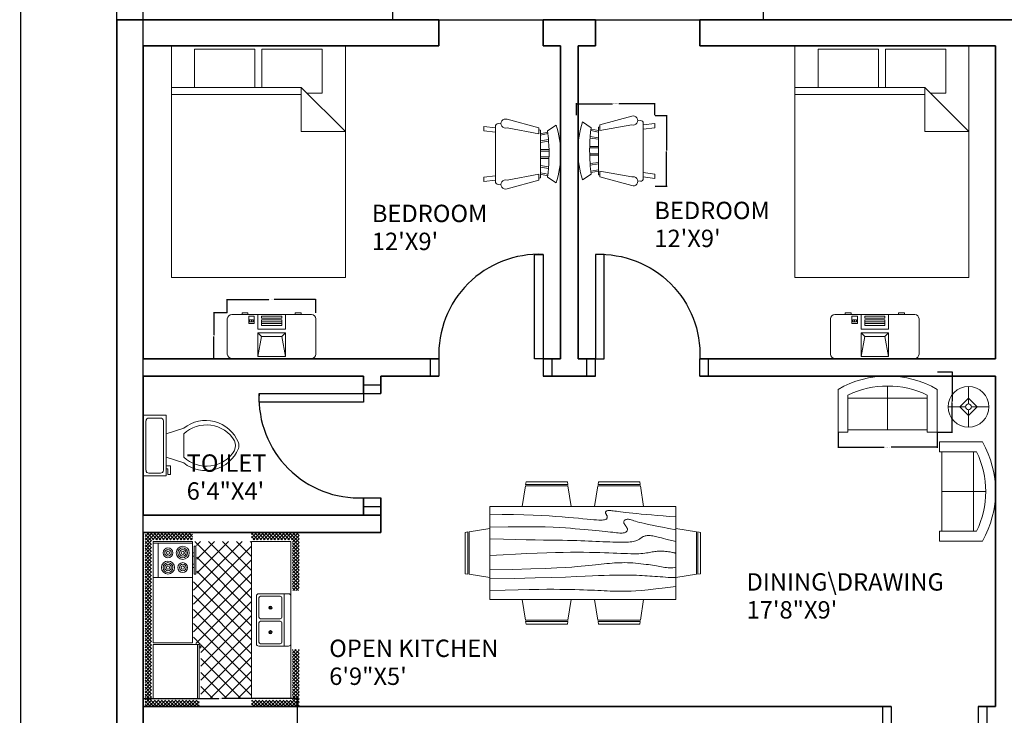
# Model space of a CAD drawing. Units: inches. Extents: x 4159 to 4826, y 299 to 1026.
# Tile 35 of 37: x 4159 to 4498, y 663 to 903. Entities that reach past the tile are written whole.
import ezdxf

# ---------------------------------------------------------------- set-up
doc = ezdxf.new("R2010")
doc.units = ezdxf.units.IN
for name, color, linetype, lineweight in [('A-ANNO-DIMS', 2, 'Continuous', 18), ('A-AREA-IDEN', 7, 'Continuous', 18), ('A-DOOR', 4, 'Continuous', 25), ('A-EQPM', 8, 'Continuous', 13), ('A-FLOR-BALC', 7, 'Continuous', 25), ('A-FLOR-FIXT', 9, 'Continuous', 18), ('A-FURN', 8, 'Continuous', 18), ('A-WALL', 7, 'Continuous', 35)]:
    doc.layers.add(name, color=color, linetype=linetype, lineweight=lineweight)
doc.styles.get("Standard").update_dxf_attribs({"font": 'arial.ttf'})
doc.dimstyles.get("Standard").update_dxf_attribs({"dimtxt": 0.18, "dimasz": 0.18, "dimexe": 0.18, "dimexo": 0.0625, "dimgap": 0.09, "dimtad": 0, "dimtih": 1, "dimtoh": 1, "dimdec": 4, "dimzin": 0, "dimdsep": 46, "dimtxsty": 'Standard', "dimcen": 0.09, "dimadec": 0, "dimazin": 0, "dimtfac": 1, "dimtdec": 4, "dimtofl": 0, "dimtmove": 0, "dimatfit": 3, "dimfxl": 1, "dimtolj": 1, "dimtzin": 0, "dimarcsym": 0})

# ---------------------------------------------------------------- blocks, each defined once
blk = doc.blocks.new('Chair - Rocking')
for p, q in [((-8, -4.5), (-10, -1.5)), ((8, -4.5), (10, -1.5)), ((-7.5, -4.5), (-7, -7)), ((-6.5, -7), (-7.02225, -4.43)), ((-4.5, -7), (-4.96674, -4.19951)), ((-4, -7), (-4.40532, -4.16272)), ((-1.5, -4.05012), (-1.5, -7)), ((-1, -7), (-1, -4.05012)), ((1, -7), (1, -4.04655)), ((1.5, -4.05012), (1.5, -7)), ((4, -7), (4.40187, -4.18694)), ((4.5, -7), (4.96761, -4.19437)), ((6.5, -7), (7, -4.4057)), ((7.5, -4.5), (7, -7)), ((-9, -7.5), (-12, -18.49999)), ((-7, -7.5), (-9, -7.5)), ((-9, -18.49999), (-7, -7.5)), ((-8.23428, -6.99939), (-8.3093, -7.47958)), ((-8.23041, -7), (8.23915, -7)), ((7, -7.5), (9, -7.5)), ((9, -18.49999), (7, -7.5)), ((8.31071, -7.48854), (8.23449, -7.00073)), ((9, -7.5), (12, -18.49999)), ((-10.36644, -20.64523), (-10.5, -21.49999)), ((-9, -22.49999), (-9.5, -26.49999)), ((0, -22.49999), (-9.5, -22.49999)), ((-8, -26.49999), (-7.5, -22.49999)), ((0, -22.49999), (9.5, -22.49999)), ((8, -26.49999), (7.5, -22.49999)), ((9, -22.49999), (9.5, -26.49999)), ((10.5, -21.49999), (10.3575, -20.58798)), ((-9.5, -26.49999), (-8, -26.49999)), ((9.5, -26.49999), (8, -26.49999))]:
    blk.add_line(p, q)
for centre, radius, start, end in [((0, -34.08333), 34.08333, 72.93847, 107.0615), ((0, -68.25004), 64.25, 93.92211, 97.15267), ((0, -68.25004), 64.25, 82.84733, 93.92211), ((-10.5, -18.99999), 1.58114, 161.5651, 18.43495), ((10.5, -18.99999), 1.58114, 161.5651, 18.43495), ((-9.5, -21.49999), 1, 180, 270), ((9.5, -21.49999), 1, 270, 0)]:
    blk.add_arc(centre, radius, start, end)
blk = doc.blocks.new('Bed - Queen')
for p, q in [((0, -80.00003), (0, 0)), ((0, 0), (59.99999, 0)), ((59.99999, 0), (59.99999, -80.00003)), ((7.99999, -1.2), (28.79998, -1.2)), ((7.99999, -14.4), (7.99999, -1.2)), ((28.79998, -1.2), (28.79998, -14.4)), ((31.19999, -1.2), (51.99999, -1.2)), ((31.19999, -14.4), (31.19999, -1.2)), ((51.99999, -1.2), (51.99999, -16.4)), ((0, -14.4), (44.8, -14.4)), ((44.8, -16.8), (0, -16.8)), ((59.99999, -29.6), (44.8, -14.4)), ((44.8, -14.4), (44.8, -29.6)), ((51.99999, -16.4), (46.79936, -16.4)), ((44.8, -29.6), (59.99999, -29.6)), ((59.99999, -80.00003), (0, -80.00003))]:
    blk.add_line(p, q)
blk = doc.blocks.new('Dining Set - 36 x 72 in.')
for p, q in [((-22, 27.5), (-22.1562, 26.50042)), ((-22, 27.5), (-6, 27.5)), ((-5.8437, 26.49966), (-6, 27.5)), ((6, 27.5), (5.8438, 26.50042)), ((6, 27.5), (22, 27.5)), ((22.1563, 26.49966), (22, 27.5)), ((-22.2343, 26.00059), (-23.4847, 17.99762)), ((-22.2304, 26), (-5.7608, 26)), ((-5.8416, 26.5), (-22.1534, 26.5)), ((-4.5152, 17.99762), (-5.7655, 25.99926)), ((5.7657, 26.00059), (4.5153, 17.99762)), ((5.7696, 26), (22.2392, 26)), ((22.1584, 26.5), (5.8466, 26.5)), ((23.4848, 17.99762), (22.2345, 25.99926)), ((36, 18), (-36, 18)), ((-36, 18), (-36, -18)), ((36, -18), (36, 18)), ((-45.5, 8), (-44.5004, 8.15617)), ((-45.5, 8), (-45.5, -8)), ((-44.5, -8.15843), (-44.5, 8.15338)), ((-44.0006, 8.23428), (-35.9976, 9.48474)), ((-44, 8.23041), (-44, -8.23915)), ((44.0006, 8.23428), (35.9976, 9.48474)), ((44, 8.23041), (44, -8.23915)), ((44.5, -8.15843), (44.5, 8.15338)), ((45.5, 8), (44.5005, 8.15617)), ((45.5, 8), (45.5, -8)), ((-44.4997, -8.15631), (-45.5, -8)), ((-35.9976, -9.48476), (-43.9993, -8.2345)), ((35.9976, -9.48476), (43.9993, -8.2345)), ((44.4997, -8.15631), (45.5, -8)), ((-36, -18), (36, -18)), ((-22.2343, -26.0006), (-23.4847, -17.99762)), ((-4.5152, -17.99762), (-5.7655, -25.99928)), ((5.7657, -26.0006), (4.5153, -17.99762)), ((23.4848, -17.99762), (22.2345, -25.99928)), ((-22.2304, -26), (-5.7608, -26)), ((-22, -27.5), (-22.1562, -26.50044)), ((-5.8416, -26.5), (-22.1534, -26.5)), ((-5.8437, -26.49967), (-6, -27.5)), ((5.7696, -26), (22.2392, -26)), ((6, -27.5), (5.8438, -26.50044)), ((22.1584, -26.5), (5.8466, -26.5)), ((22.1563, -26.49967), (22, -27.5)), ((-22, -27.5), (-6, -27.5)), ((6, -27.5), (22, -27.5))]:
    blk.add_line(p, q)
for points in [[(-36, 15), (-31.1772, 14.97754), (-26.8079, 14.91406), (-22.8538, 14.81543), (-19.276, 14.6875), (-16.0362, 14.53613), (-13.0957, 14.36718), (-10.4159, 14.18652), (-7.9583, 14), (-5.6904, 13.81315), (-3.6035, 13.63021), (-1.6954, 13.45508), (0.0365, 13.29166), (1.5945, 13.14388), (2.9811, 13.01562), (4.1988, 12.9108), (5.25, 12.83333), (6.1393, 12.78613), (6.8802, 12.76823), (7.4883, 12.77767), (7.9792, 12.8125), (8.3685, 12.87077), (8.6719, 12.95052), (8.9049, 13.0498), (9.0833, 13.16666), (9.2205, 13.29899), (9.3216, 13.44401), (9.3895, 13.59879), (9.4271, 13.76041), (9.4373, 13.92594), (9.4232, 14.09245), (9.3875, 14.257), (9.3333, 14.41666), (9.2638, 14.56917), (9.1836, 14.71484), (9.0975, 14.85465), (9.0104, 14.98958), (8.9272, 15.1206), (8.8529, 15.2487), (8.7922, 15.37483), (8.75, 15.5), (8.7305, 15.62467), (8.7344, 15.74739), (8.7617, 15.86621), (8.8125, 15.97916), (8.8867, 16.08431), (8.9844, 16.17968), (9.1055, 16.26334), (9.25, 16.33333), (9.4189, 16.38802), (9.6172, 16.42708), (9.8506, 16.45052), (10.125, 16.45833), (10.4463, 16.45052), (10.8203, 16.42708), (11.2529, 16.38802), (11.75, 16.33333), (12.3184, 16.26318), (12.9694, 16.17838), (13.7151, 16.07991), (14.5677, 15.96875), (15.5395, 15.84586), (16.6426, 15.71224), (17.8893, 15.56884), (19.2917, 15.41666), (20.859, 15.25667), (22.5879, 15.08984), (24.4721, 14.91715), (26.5052, 14.73958), (28.6809, 14.5581), (30.9929, 14.3737), (33.4347, 14.18733), (36, 14)], [(-36, 10), (-28.9766, 10.14274), (-23.1725, 10.20442), (-18.4241, 10.19775), (-14.5677, 10.13541), (-11.4399, 10.03011), (-8.877, 9.89453), (-6.7154, 9.74137), (-4.7917, 9.58333), (-2.9698, 9.43082), (-1.2246, 9.28515), (0.4415, 9.14534), (2.026, 9.01041), (3.5266, 8.87939), (4.9408, 8.7513), (6.266, 8.62516), (7.5, 8.5), (8.6411, 8.37549), (9.6914, 8.2539), (10.6538, 8.13818), (11.5312, 8.03125), (12.3267, 7.93603), (13.043, 7.85547), (13.6831, 7.79248), (14.25, 7.75), (14.7471, 7.7303), (15.1797, 7.73307), (15.5537, 7.75732), (15.875, 7.80208), (16.1494, 7.86637), (16.3828, 7.94922), (16.5811, 8.04964), (16.75, 8.16666), (16.8944, 8.29915), (17.0143, 8.44531), (17.1089, 8.60319), (17.1771, 8.77083), (17.218, 8.94629), (17.2305, 9.1276), (17.2137, 9.31282), (17.1667, 9.5), (17.0895, 9.6875), (16.987, 9.875), (16.8649, 10.0625), (16.7292, 10.25), (16.5856, 10.4375), (16.4401, 10.625), (16.2985, 10.8125), (16.1667, 11), (16.05, 11.18733), (15.9518, 11.3737), (15.8752, 11.5581), (15.8229, 11.73958), (15.798, 11.91715), (15.8034, 12.08984), (15.842, 12.25667), (15.9167, 12.41666), (16.0295, 12.56836), (16.1784, 12.70833), (16.3605, 12.83268), (16.5729, 12.9375), (16.8127, 13.01888), (17.0768, 13.07291), (17.3625, 13.0957), (17.6667, 13.08333), (17.9894, 13.03312), (18.3418, 12.94726), (18.7382, 12.82918), (19.1927, 12.68229), (19.7195, 12.51001), (20.3327, 12.31575), (21.0465, 12.10294), (21.875, 11.875), (22.8357, 11.63354), (23.959, 11.37304), (25.2786, 11.08618), (26.8282, 10.76562), (28.6414, 10.40405), (30.752, 9.99414), (33.1936, 9.52856), (36, 9)], [(-36, 5.5), (-30.7157, 5.3348), (-26.069, 5.20963), (-21.9946, 5.11767), (-18.4271, 5.05208), (-15.3009, 5.00602), (-12.5508, 4.97265), (-10.1112, 4.94515), (-7.9167, 4.91666), (-5.909, 4.88167), (-4.0586, 4.83984), (-2.3429, 4.79215), (-0.7396, 4.73958), (0.7739, 4.6831), (2.22, 4.6237), (3.6213, 4.56233), (5, 4.5), (6.373, 4.43782), (7.7344, 4.3776), (9.0723, 4.32129), (10.375, 4.27083), (11.6309, 4.22819), (12.8281, 4.19531), (13.9551, 4.17415), (15, 4.16666), (15.954, 4.17448), (16.819, 4.19791), (17.6001, 4.23698), (18.3021, 4.29166), (18.9299, 4.36198), (19.4883, 4.44791), (19.9823, 4.54948), (20.4167, 4.66666), (20.7969, 4.79899), (21.1302, 4.94401), (21.4245, 5.09879), (21.6875, 5.26041), (21.9271, 5.42594), (22.1511, 5.59245), (22.3672, 5.757), (22.5834, 5.91666), (22.8065, 6.06868), (23.0404, 6.21093), (23.2879, 6.34147), (23.5521, 6.45833), (23.8358, 6.55957), (24.142, 6.64323), (24.4735, 6.70735), (24.8334, 6.75), (25.2235, 6.76969), (25.642, 6.76692), (26.0858, 6.74267), (26.5521, 6.69791), (27.0379, 6.63362), (27.5404, 6.55078), (28.0565, 6.45036), (28.5834, 6.33333), (29.1242, 6.19987), (29.7071, 6.04687), (30.3661, 5.87044), (31.1354, 5.66666), (32.0493, 5.43164), (33.142, 5.16146), (34.4475, 4.85221), (36, 4.5)], [(-36, -1), (-30.7915, -0.6591), (-26.0195, -0.38216), (-21.6519, -0.16284), (-17.6563, 0.00521), (-14.0005, 0.12833), (-10.6523, 0.21289), (-7.5796, 0.26522), (-4.75, 0.29166), (-2.134, 0.29793), (0.2878, 0.28711), (2.5317, 0.26163), (4.6146, 0.22396), (6.5529, 0.17651), (8.3633, 0.12174), (10.0623, 0.06209), (11.6667, 0), (13.1899, -0.06201), (14.6341, -0.1211), (15.9982, -0.17432), (17.2813, -0.21875), (18.4823, -0.25147), (19.6003, -0.26953), (20.6343, -0.27002), (21.5834, -0.25), (22.4481, -0.20768), (23.2357, -0.14584), (23.9549, -0.06836), (24.6146, 0.02083), (25.2235, 0.11784), (25.7904, 0.21875), (26.3241, 0.31966), (26.8334, 0.41666), (27.3265, 0.50618), (27.8099, 0.58593), (28.2894, 0.65397), (28.7709, 0.70833), (29.2601, 0.74707), (29.763, 0.76823), (30.2855, 0.76985), (30.8334, 0.75), (31.4088, 0.70784), (31.9994, 0.64713), (32.589, 0.57275), (33.1615, 0.48958), (33.7008, 0.4025), (34.1908, 0.3164), (34.6153, 0.23616), (34.9584, 0.16666), (35.2099, 0.11165), (35.3848, 0.07031), (35.504, 0.04069), (35.5886, 0.02083), (35.6594, 0.00879), (35.7377, 0.0026), (35.8442, 0.00032), (36, 0)], [(-36, -6.5), (-27.1843, -6.31267), (-20.084, -6.1263), (-14.469, -5.9419), (-10.1094, -5.76042), (-6.7752, -5.58285), (-4.2363, -5.41016), (-2.2629, -5.24333), (-0.625, -5.08334), (0.8708, -4.93099), (2.2715, -4.78646), (3.5872, -4.64974), (4.8281, -4.52084), (6.0046, -4.39974), (7.127, -4.28646), (8.2053, -4.18099), (9.25, -4.08334), (10.2705, -3.99382), (11.2734, -3.91407), (12.2647, -3.84603), (13.25, -3.79167), (14.2354, -3.75293), (15.2266, -3.73177), (16.2295, -3.73015), (17.25, -3.75), (18.2912, -3.79248), (19.3451, -3.85547), (20.4009, -3.93604), (21.4479, -4.03125), (22.4754, -4.13819), (23.4727, -4.25391), (24.4289, -4.37549), (25.3334, -4.5), (26.1785, -4.62492), (26.9694, -4.74935), (27.7145, -4.87281), (28.4219, -4.99479), (29.1, -5.11483), (29.7572, -5.23242), (30.4016, -5.34709), (31.0417, -5.45834), (31.6837, -5.56437), (32.3262, -5.65821), (32.9658, -5.73153), (33.599, -5.77604), (34.2224, -5.78345), (34.8327, -5.74545), (35.4264, -5.65373), (36, -5.5)], [(-36, -10), (-26.4022, -9.81299), (-18.4675, -9.62891), (-11.9839, -9.45069), (-6.7396, -9.28125), (-2.5226, -9.12354), (0.8789, -8.98047), (3.6769, -8.85498), (6.0833, -8.75), (8.2767, -8.66765), (10.3021, -8.60677), (12.1712, -8.56543), (13.8958, -8.54167), (15.4876, -8.53353), (16.9583, -8.53907), (18.3197, -8.55632), (19.5834, -8.58334), (20.7616, -8.61841), (21.8685, -8.66081), (22.9188, -8.71004), (23.9271, -8.76563), (24.9081, -8.82707), (25.8763, -8.89388), (26.8465, -8.96558), (27.8334, -9.04167), (28.8474, -9.12118), (29.8828, -9.20117), (30.93, -9.27824), (31.9792, -9.34896), (33.0205, -9.40991), (34.0443, -9.45768), (35.0407, -9.48885), (36, -9.5)], [(-36, -14.5), (-30.0881, -14.33513), (-25.0332, -14.21224), (-20.7312, -14.12647), (-17.0781, -14.07292), (-13.97, -14.04671), (-11.3027, -14.04297), (-8.9724, -14.05681), (-6.875, -14.08334), (-4.9224, -14.11833), (-3.0905, -14.16016), (-1.3709, -14.20785), (0.2448, -14.26042), (1.7647, -14.3169), (3.1973, -14.3763), (4.5507, -14.43767), (5.8333, -14.5), (7.0554, -14.5621), (8.235, -14.62175), (9.3922, -14.67652), (10.5469, -14.72396), (11.7192, -14.76164), (12.929, -14.78711), (14.1965, -14.79794), (15.5417, -14.79167), (16.9933, -14.76424), (18.6152, -14.70508), (20.4804, -14.60197), (22.6615, -14.44271), (25.2312, -14.21509), (28.2624, -13.9069), (31.8277, -13.50594), (36, -13)]]:
    blk.add_lwpolyline(points)
blk = doc.blocks.new('Sofa - Roundback Loveseat 5 ft.')
for p, q in [((-24, -33.99998), (-24, -11.46958)), ((0, -32.44198), (0, -5.99998)), ((24.00004, -33.99998), (24.00004, -11.46958)), ((-23.9998, -13.38178), (23.99986, -13.38178)), ((-24, -32.44198), (24.00004, -32.44198))]:
    blk.add_line(p, q)
for points in [[(-24, -33.99998), (-30, -33.99998), (-30, -7.99998)], [(30.00004, -7.99998), (30.00004, -33.99998), (24.00004, -33.99998)]]:
    blk.add_lwpolyline(points)
for centre, radius, start, end in [((0, -60.24998), 60.24998, 60.13715, 119.8628), ((0, -61.38438), 55.38444, 64.32083, 115.6792)]:
    blk.add_arc(centre, radius, start, end)
blk = doc.blocks.new('Toilet - top')
for p, q in [((9.5, -6), (9.5, -2)), ((-10, -8.5), (-8, -8.5)), ((-10, -9.5), (-10, -8.5)), ((-7, -9.5), (-10, -9.5)), ((-8, -8.5), (-8, -8)), ((-7, -8), (-7, -9.5)), ((-4, -8), (-6, -14)), ((4, -8), (6, -14)), ((4, -14), (-4, -14))]:
    blk.add_line(p, q)
blk.add_lwpolyline([(10.5, -8), (10.5, 0), (-10.5, 0), (-10.5, -8)], close=True)
for points in [[(-9.5, -2), (-9.5, -6)], [(8.5, -1), (-8.5, -1)], [(-8.5, -7), (8.5, -7)]]:
    blk.add_lwpolyline(points)
for centre, radius, start, end in [((-8.62, -1.88), 0.884, 81.8699, 188.1301), ((8.62, -1.88), 0.884, 351.8699, 98.1301), ((-8.62, -6.12), 0.884, 171.8699, 278.1301), ((8.62, -6.12), 0.884, 261.8699, 8.1301), ((3.52, -21.58), 12.17, 141.4691, 247.9714), ((4.2, -21.82), 11.33, 136.3677, 238.9468), ((-3.52, -21.58), 12.17, 292.0284, 38.5307), ((-4.2, -21.82), 11.33, 301.053, 43.6321), ((0, -27.88), 4, 245.7318, 294.2682), ((0, -29), 4, 254.8605, 285.1395)]:
    blk.add_arc(centre, radius, start, end)
blk = doc.blocks.new('Lamp - Table')
for p, q in [((0, 7), (0, 1)), ((-1, 0), (-7, 0)), ((0, 3), (-3, 0)), ((-3, 0), (0, -3)), ((3, 0), (0, 3)), ((0, -3), (3, 0)), ((1, 0), (7, 0)), ((0, -1), (0, -7))]:
    blk.add_line(p, q)
for radius in [7, 1]:
    blk.add_circle((0, 0), radius)
blk = doc.blocks.new('Kitchen Layout - 7 x 8 ft')
for p, q in [((-5, 81.32), (2.68, 89)), ((-5, 83.44), (0.56, 89)), ((-5, 85.56), (-1.56, 89)), ((-5, 87.68), (-3.68, 89)), ((-1, 84.97), (-5, 88.97)), ((-1, 82.85), (-5, 86.85)), ((-1, 80.73), (-5, 84.73)), ((1.09, 85), (-2.91, 89)), ((3.21, 85), (-0.79, 89)), ((0.81, 85), (4.81, 89)), ((5.34, 85), (1.34, 89)), ((2.93, 85), (6.93, 89)), ((7.46, 85), (3.46, 89)), ((5.05, 85), (9.05, 89)), ((9.58, 85), (5.58, 89)), ((7.17, 85), (11.17, 89)), ((11.7, 85), (7.7, 89)), ((9.29, 85), (13.29, 89)), ((13.82, 85), (9.82, 89)), ((11.41, 85), (15.41, 89)), ((15.94, 85), (11.94, 89)), ((13.53, 85), (17.53, 89)), ((18.06, 85), (14.06, 89)), ((15.65, 85), (19.65, 89)), ((20.18, 85), (16.18, 89)), ((17.78, 85), (21.78, 89)), ((22.31, 85), (18.31, 89)), ((19.9, 85), (23.9, 89)), ((24.43, 85), (20.43, 89)), ((22.02, 85), (26.02, 89)), ((26.55, 85), (22.55, 89)), ((24.14, 85), (28.14, 89)), ((28.67, 85), (24.67, 89)), ((26.26, 85), (30.26, 89)), ((30.79, 85), (26.79, 89)), ((28.38, 85), (32.38, 89)), ((32.91, 85), (28.91, 89)), ((30.5, 85), (34.5, 89)), ((35.03, 85), (31.03, 89)), ((32.63, 85), (36.63, 89)), ((37.16, 85), (33.16, 89)), ((34.75, 85), (38.75, 89)), ((39.28, 85), (35.28, 89)), ((36.87, 85), (40.87, 89)), ((41.4, 85), (37.4, 89)), ((38.99, 85), (42.99, 89)), ((43.52, 85), (39.52, 89)), ((41.11, 85), (45.11, 89)), ((45.64, 85), (41.64, 89)), ((43.23, 85), (47.23, 89)), ((47.76, 85), (43.76, 89)), ((45.35, 85), (49.35, 89)), ((49.88, 85), (45.88, 89)), ((47.47, 85), (51.47, 89)), ((52, 85), (48, 89)), ((49.6, 85), (53.6, 89)), ((54.13, 85), (50.13, 89)), ((51.72, 85), (55.72, 89)), ((56.25, 85), (52.25, 89)), ((53.84, 85), (57.84, 89)), ((58.37, 85), (54.37, 89)), ((55.96, 85), (59.96, 89)), ((60.49, 85), (56.49, 89)), ((58.08, 85), (62.08, 89)), ((62.61, 85), (58.61, 89)), ((60.2, 85), (64.2, 89)), ((64.73, 85), (60.73, 89)), ((62.32, 85), (66.32, 89)), ((66.85, 85), (62.85, 89)), ((64.45, 85), (68.45, 89)), ((68.97, 85), (64.97, 89)), ((66.57, 85), (70.57, 89)), ((71.1, 85), (67.1, 89)), ((68.69, 85), (72.69, 89)), ((73.22, 85), (69.22, 89)), ((70.81, 85), (74.81, 89)), ((75.34, 85), (71.34, 89)), ((72.93, 85), (76.93, 89)), ((77.46, 85), (73.46, 89)), ((75.05, 85), (79.05, 89)), ((79.58, 85), (75.58, 89)), ((77.17, 85), (81.17, 89)), ((81.7, 85), (77.7, 89)), ((79.29, 85), (83.29, 89)), ((83.82, 85), (79.82, 89)), ((81.42, 85), (85.42, 89)), ((85.95, 85), (81.95, 89)), ((83.54, 85), (87.54, 89)), ((88.07, 85), (84.07, 89)), ((85.66, 85), (89.66, 89)), ((90.19, 85), (86.19, 89)), ((87.78, 85), (91.78, 89)), ((92.31, 85), (88.31, 89)), ((89.9, 85), (93.9, 89)), ((94.43, 85), (90.43, 89)), ((92.02, 85), (96.02, 89)), ((96.55, 85), (92.55, 89)), ((94.14, 85), (98.14, 89)), ((101, 82.67), (94.67, 89)), ((96.27, 85), (100.27, 89)), ((101, 84.79), (96.79, 89)), ((97, 83.61), (101, 87.61)), ((97, 81.49), (101, 85.49)), ((101, 80.55), (97, 84.55)), ((101, 86.92), (98.92, 89)), ((-5, 79.19), (-1, 83.19)), ((-1, 78.61), (-5, 82.61)), ((-5, 77.07), (-1, 81.07)), ((-1, 76.49), (-5, 80.49)), ((-5, 74.95), (-1, 78.95)), ((-1, 74.36), (-5, 78.36)), ((34, 84), (96, 84)), ((34, 60), (34, 84)), ((74, 81), (95, 81)), ((96, 84), (96, 60)), ((97, 79.37), (101, 83.37)), ((101, 78.43), (97, 82.43)), ((97, 77.25), (101, 81.25)), ((101, 76.31), (97, 80.31)), ((97, 75.13), (101, 79.13)), ((101, 74.19), (97, 78.19)), ((-5, 72.83), (-1, 76.83)), ((-1, 72.24), (-5, 76.24)), ((-5, 70.71), (-1, 74.71)), ((-1, 70.12), (-5, 74.12)), ((-5, 68.59), (-1, 72.59)), ((97, 73.01), (101, 77.01)), ((101, 72.07), (97, 76.07)), ((97, 70.89), (101, 74.89)), ((101, 69.95), (97, 73.95)), ((97, 68.76), (101, 72.76)), ((-1, 68), (-5, 72)), ((-5, 66.47), (-1, 70.47)), ((-1, 65.88), (-5, 69.88)), ((-5, 64.35), (-1, 68.35)), ((-1, 63.76), (-5, 67.76)), ((-5, 62.22), (-1, 66.22)), ((101, 67.82), (97, 71.82)), ((97, 66.64), (101, 70.64)), ((101, 65.7), (97, 69.7)), ((97, 64.52), (101, 68.52)), ((101, 63.58), (97, 67.58)), ((97, 62.4), (101, 66.4)), ((-1, 61.64), (-5, 65.64)), ((-5, 60.1), (-1, 64.1)), ((-1, 59.52), (-5, 63.52)), ((-5, 57.98), (-1, 61.98)), ((-1, 57.39), (-5, 61.39)), ((101, 61.46), (97, 65.46)), ((97, 60.28), (101, 64.28)), ((100.34, 60), (97, 63.34)), ((98.22, 60), (97, 61.22)), ((98.84, 60), (101, 62.16)), ((-1.73, 56), (-5, 59.27)), ((-3.85, 56), (-5, 57.15)), ((-4.86, 56), (-1, 59.86)), ((-2.74, 56), (-1, 57.74)), ((0, 57), (33, 57)), ((0, 30.57), (24.43, 55)), ((0, 39.06), (15.94, 55)), ((0, 47.54), (7.46, 55)), ((1.91, 24), (32.91, 55)), ((33.77, 24), (2.77, 55)), ((10.4, 24), (45.9, 59.5)), ((42.26, 24), (11.26, 55)), ((18.88, 24), (54.38, 59.5)), ((50.74, 24), (19.74, 55)), ((27.37, 24), (62.87, 59.5)), ((59.23, 24), (28.23, 55)), ((31, 55), (31, 56)), ((32, 55), (31, 55)), ((32, 56), (32, 55)), ((33.03, 55.11), (37.41, 59.5)), ((67.71, 24), (33.68, 58.04)), ((96, 60), (34, 60)), ((35.85, 24), (71.35, 59.5)), ((76.2, 24), (40.7, 59.5)), ((44.34, 24), (77.84, 57.5)), ((84.68, 24), (49.18, 59.5)), ((52.82, 24), (86.32, 57.5)), ((93.17, 24), (57.67, 59.5)), ((61.31, 24), (96, 58.69)), ((96, 29.65), (66.15, 59.5)), ((96, 38.14), (76.64, 57.5)), ((80, 60), (80, 59)), ((82, 59), (82, 60)), ((96, 46.63), (85.13, 57.5)), ((87, 59), (87, 60)), ((89, 60), (89, 59)), ((96, 55.11), (93.57, 57.54)), ((100.96, 60), (101, 60.04)), ((25.29, 24), (0, 49.29)), ((69.79, 24), (96, 50.21)), ((16.8, 24), (0, 40.8)), ((78.28, 24), (96, 41.72)), ((8.32, 24), (0, 32.32)), ((86.76, 24), (96, 33.24)), ((95.25, 24), (96, 24.75)), ((-5, 21.92), (-2.92, 24)), ((-5, 19.8), (-1, 23.8)), ((-1, 19.21), (-5, 23.21)), ((-5, 17.68), (-1, 21.68)), ((-1, 17.09), (-5, 21.09)), ((-5, 15.55), (-1, 19.55)), ((-1, 14.97), (-5, 18.97)), ((-1, 21.33), (-3.67, 24)), ((-1, 23.45), (-1.55, 24)), ((0, 24), (96, 24)), ((0, 0), (0, 24)), ((47.25, 6.5), (47.25, 18.5)), ((48.75, 18.5), (48.75, 6.5)), ((96, 24), (96, 0)), ((97, 22.1), (98.9, 24)), ((97, 19.97), (101, 23.97)), ((101, 19.03), (97, 23.03)), ((97, 17.85), (101, 21.85)), ((101, 16.91), (97, 20.91)), ((97, 15.73), (101, 19.73)), ((101, 14.79), (97, 18.79)), ((101, 21.16), (98.16, 24)), ((101, 23.28), (100.28, 24)), ((-5, 13.43), (-1, 17.43)), ((-1, 12.85), (-5, 16.85)), ((-5, 11.31), (-1, 15.31)), ((-1, 10.73), (-5, 14.73)), ((-5, 9.19), (-1, 13.19)), ((-1, 8.6), (-5, 12.6)), ((97, 13.61), (101, 17.61)), ((101, 12.67), (97, 16.67)), ((97, 11.49), (101, 15.49)), ((101, 10.55), (97, 14.55)), ((97, 9.37), (101, 13.37)), ((101, 8.43), (97, 12.43)), ((-5, 7.07), (-1, 11.07)), ((-1, 6.48), (-5, 10.48)), ((-5, 4.95), (-1, 8.95)), ((-1, 4.36), (-5, 8.36)), ((-5, 2.83), (-1, 6.83)), ((-1, 2.24), (-5, 6.24)), ((97, 7.25), (101, 11.25)), ((101, 6.31), (97, 10.31)), ((97, 5.12), (101, 9.12)), ((101, 4.18), (97, 8.18)), ((97, 3), (101, 7)), ((101, 2.06), (97, 6.06)), ((-5, 0.71), (-1, 4.71)), ((-1, 0.12), (-5, 4.12)), ((-5, -1.42), (-1, 2.58)), ((2, -5), (-5, 2)), ((-5, -3.54), (-1, 0.46)), ((96, 0), (0, 0)), ((64, 4), (32, 4)), ((93.24, -5), (101, 2.76)), ((95.36, -5), (101, 0.64)), ((97, 0.88), (101, 4.88)), ((101, -0.06), (97, 3.94)), ((101, -2.18), (97, 1.82)), ((-0.12, -5), (-5, -0.12)), ((-2.25, -5), (-5, -2.25)), ((-4.37, -5), (-5, -4.37)), ((-4.34, -5), (-0.34, -1)), ((-2.22, -5), (1.78, -1)), ((-0.1, -5), (3.9, -1)), ((4.12, -5), (0.12, -1)), ((2.02, -5), (6.02, -1)), ((6.24, -5), (2.24, -1)), ((4.14, -5), (8.14, -1)), ((8.36, -5), (4.36, -1)), ((6.27, -5), (10.27, -1)), ((10.48, -5), (6.48, -1)), ((8.39, -5), (12.39, -1)), ((12.6, -5), (8.6, -1)), ((10.51, -5), (14.51, -1)), ((14.73, -5), (10.73, -1)), ((12.63, -5), (16.63, -1)), ((16.85, -5), (12.85, -1)), ((14.75, -5), (18.75, -1)), ((18.97, -5), (14.97, -1)), ((16.87, -5), (20.87, -1)), ((21.09, -5), (17.09, -1)), ((18.99, -5), (22.99, -1)), ((23.21, -5), (19.21, -1)), ((21.11, -5), (25.11, -1)), ((25.33, -5), (21.33, -1)), ((23.24, -5), (27.24, -1)), ((27.45, -5), (23.45, -1)), ((25.36, -5), (29.36, -1)), ((29.57, -5), (25.57, -1)), ((27.48, -5), (30, -2.48)), ((30, -3.3), (27.7, -1)), ((29.6, -5), (30, -4.6)), ((30, -1.18), (29.82, -1)), ((66, -2.54), (67.54, -1)), ((66, -4.66), (69.66, -1)), ((69.88, -5), (66, -1.12)), ((67.76, -5), (66, -3.24)), ((67.78, -5), (71.78, -1)), ((72, -5), (68, -1)), ((69.9, -5), (73.9, -1)), ((74.12, -5), (70.12, -1)), ((72.03, -5), (76.03, -1)), ((76.24, -5), (72.24, -1)), ((74.15, -5), (78.15, -1)), ((78.36, -5), (74.36, -1)), ((76.27, -5), (80.27, -1)), ((80.49, -5), (76.49, -1)), ((78.39, -5), (82.39, -1)), ((82.61, -5), (78.61, -1)), ((80.51, -5), (84.51, -1)), ((84.73, -5), (80.73, -1)), ((82.63, -5), (86.63, -1)), ((86.85, -5), (82.85, -1)), ((84.75, -5), (88.75, -1)), ((88.97, -5), (84.97, -1)), ((86.88, -5), (90.88, -1)), ((91.09, -5), (87.09, -1)), ((89, -5), (93, -1)), ((93.21, -5), (89.21, -1)), ((91.12, -5), (95.12, -1)), ((95.34, -5), (91.34, -1)), ((97.46, -5), (93.46, -1)), ((99.58, -5), (95.58, -1)), ((101, -4.3), (97, -0.3)), ((97.48, -5), (101, -1.48)), ((99.6, -5), (101, -3.6))]:
    blk.add_line(p, q)
for points in [[(0, 56), (0, 84), (33, 84), (33, 56)], [(74, 60), (74, 84), (95, 84), (95, 60)], [(76, 58), (76, 59), (93, 59), (93, 58)]]:
    blk.add_lwpolyline(points, close=True)
for points in [[(32, 1.5), (32, 19.5)], [(33.5, 21), (62.5, 21)], [(33.5, 6.5), (33.5, 18.5)], [(34.5, 19.5), (46.25, 19.5)], [(49.75, 19.5), (61.5, 19.5)], [(62.5, 18.5), (62.5, 6.5)], [(64, 19.5), (64, 1.5)], [(62.5, 0), (33.5, 0)], [(46.25, 5.5), (34.5, 5.5)], [(61.5, 5.5), (49.75, 5.5)]]:
    blk.add_lwpolyline(points)
for centre, radius in [((80, 75), 4), ((80, 75), 3), ((80, 75), 2), ((80, 75), 1), ((89, 75), 3), ((89, 75), 2), ((89, 75), 1), ((80, 66), 3), ((80, 66), 2), ((80, 66), 1), ((89, 66), 4), ((89, 66), 3), ((89, 66), 2), ((89, 66), 1), ((40.5, 12.5), 1), ((40.5, 12.5), 0.5), ((55.5, 12.5), 1), ((55.5, 12.5), 0.5)]:
    blk.add_circle(centre, radius)
for centre, radius, start, end in [((33.5, 19.5), 1.5, 90, 180), ((34.5, 18.5), 1, 90, 180), ((46.25, 18.5), 1, 0, 90), ((49.75, 18.5), 1, 90, 180), ((61.5, 18.5), 1, 0, 90), ((62.5, 19.5), 1.5, 0, 90), ((34.5, 6.5), 1, 180, 270), ((46.25, 6.5), 1, 270, 0), ((49.75, 6.5), 1, 180, 270), ((61.5, 6.5), 1, 270, 0), ((33.5, 1.5), 1.5, 180, 270), ((62.5, 1.5), 1.5, 270, 0)]:
    blk.add_arc(centre, radius, start, end)
blk = doc.blocks.new('Desk - 30 x 60 in.')
for p, q in [((-26.999995, 0), (26.999995, 0)), ((-29.999995, -27), (-29.999995, -3)), ((29.999995, -3), (29.999995, -27)), ((26.999995, -30), (-26.999995, -30)), ((-20.000005, -30), (-20.000005, -31)), ((-20.000005, -31), (-16.000005, -31)), ((-16.000005, -31), (-16.000005, -30)), ((15.999995, -31), (15.999995, -30)), ((19.999995, -31), (15.999995, -31)), ((19.999995, -30), (19.999995, -31))]:
    blk.add_line(p, q)
for centre, start, end in [((-26.499995, -3.5), 98.1301, 171.8699), ((26.499995, -3.5), 8.130102, 81.8699), ((-26.499995, -26.5), 188.1301, 261.8699), ((26.499995, -26.5), 278.1301, 351.8699)]:
    blk.add_arc(centre, 3.535534, start, end)
blk = doc.blocks.new('Computer Terminal')
for p, q in [((-10, 11.5), (5, 11.5)), ((-8, 0.5), (-10, 11.5)), ((-10, -1.5), (-10, 11.5)), ((5, 11.5), (3, 0.5)), ((5, 11.5), (5, -1.5)), ((-10, -1.5), (-8, 0.5)), ((3, 0.5), (-8, 0.5)), ((3, 0.5), (5, -1.5)), ((5, -1.5), (-10, -1.5)), ((-10, -11.5), (-10, -3.5)), ((-10, -3.5), (5, -3.5)), ((5, -3.5), (5, -11.5)), ((-8, -5.5), (-8, -8.5)), ((3, -5.5), (-8, -5.5)), ((3, -6.5), (-8, -6.5)), ((-8, -7.5), (3, -7.5)), ((-8, -8.5), (3, -8.5)), ((-8, -9.5), (-8, -10.5)), ((3, -9.5), (-8, -9.5)), ((-8, -10.5), (3, -10.5)), ((3, -8.5), (3, -5.5)), ((3, -10.5), (3, -9.5)), ((10, -6.5), (7, -6.5)), ((7, -6.5), (7, -10.5)), ((7, -10.5), (10, -10.5)), ((9.5, -7.5), (7.5, -7.5)), ((7.5, -7.5), (7.5, -8.5)), ((7.5, -8.5), (9.5, -8.5)), ((8.5, -7.5), (8.5, -8.5)), ((9.5, -8.5), (9.5, -7.5)), ((10, -10.5), (10, -6.5)), ((5, -11.5), (-10, -11.5))]:
    blk.add_line(p, q)
blk = doc.blocks.new('DOOR-SWING-36IN')
blk.add_lwpolyline([(0, 0), (-3, 0), (-3, 36), (0, 36)], close=True)
blk.add_arc((-1.5, 1.5), 34.53, 87.5104, 182.4896)
blk = doc.blocks.new('DOOR-FRAME-36IN')
for p, q in [((0, 6), (0, 0)), ((3, 6), (3, 0)), ((39, 6), (39, 0)), ((42, 6), (42, 0))]:
    blk.add_line(p, q)
blk = doc.blocks.new('DOOR-FRAME-30IN')
for p, q in [((0, 6), (0, 0)), ((3, 6), (3, 0)), ((33, 6), (33, 0)), ((36, 6), (36, 0))]:
    blk.add_line(p, q)
blk = doc.blocks.new('*D25')
at = {"layer": 'A-ANNO-DIMS', "color": 0, "lineweight": -2, "transparency": 16777216}
for p, q in [((4440.97, 760.81), (4440.97, 755.56)), ((4475.17, 760.81), (4475.17, 755.56)), ((4441.15, 755.74), (4456.85, 755.74)), ((4474.99, 755.74), (4459.29, 755.74))]:
    blk.add_line(p, q, dxfattribs=at)
at = {"layer": 'A-ANNO-DIMS', "color": 0, "transparency": 16777216}
for points in [[(4441.15, 755.77), (4441.15, 755.71), (4440.97, 755.74)], [(4474.99, 755.77), (4474.99, 755.71), (4475.17, 755.74)]]:
    blk.add_solid(points, dxfattribs=at)
at = {"layer": 'Defpoints', "color": 0, "transparency": 16777216}
for p in [(4440.97, 760.87), (4475.17, 760.87), (4475.17, 755.74)]:
    blk.add_point(p, dxfattribs=at)
at = {"layer": 'A-ANNO-DIMS', "color": 0, "transparency": 16777216, "insert": (4458.07, 755.74), "char_height": 0.18, "attachment_point": 5}
blk.add_mtext('\\A1;LOVESEAT 34 TYP.', dxfattribs=at)
blk = doc.blocks.new('*D26')
at = {"layer": 'A-ANNO-DIMS', "color": 0, "lineweight": -2, "transparency": 16777216}
for p, q in [((4475.23, 781.77), (4480.48, 781.77)), ((4480.3, 781.59), (4480.3, 771.5)), ((4480.3, 761.05), (4480.3, 771.14)), ((4475.23, 760.87), (4480.48, 760.87))]:
    blk.add_line(p, q, dxfattribs=at)
at = {"layer": 'A-ANNO-DIMS', "color": 0, "transparency": 16777216}
for points in [[(4480.27, 781.59), (4480.33, 781.59), (4480.3, 781.77)], [(4480.27, 761.05), (4480.33, 761.05), (4480.3, 760.87)]]:
    blk.add_solid(points, dxfattribs=at)
at = {"layer": 'Defpoints', "color": 0, "transparency": 16777216}
for p in [(4475.17, 781.77), (4480.3, 781.77), (4475.17, 760.87)]:
    blk.add_point(p, dxfattribs=at)
at = {"layer": 'A-ANNO-DIMS', "color": 0, "transparency": 16777216, "insert": (4480.3, 771.32), "char_height": 0.18, "attachment_point": 5}
blk.add_mtext('\\A1;21 TYP.', dxfattribs=at)
blk = doc.blocks.new('*D27')
at = {"layer": 'A-ANNO-DIMS', "color": 0, "lineweight": -2, "transparency": 16777216}
for p, q in [((4230.34, 802.12), (4230.34, 806.83)), ((4230.52, 806.65), (4244.73, 806.65)), ((4260.75, 806.65), (4246.53, 806.65)), ((4260.93, 802.12), (4260.93, 806.83))]:
    blk.add_line(p, q, dxfattribs=at)
at = {"layer": 'A-ANNO-DIMS', "color": 0, "transparency": 16777216}
for points in [[(4230.52, 806.68), (4230.52, 806.62), (4230.34, 806.65)], [(4260.75, 806.68), (4260.75, 806.62), (4260.93, 806.65)]]:
    blk.add_solid(points, dxfattribs=at)
at = {"layer": 'Defpoints', "color": 0, "transparency": 16777216}
for p in [(4230.34, 806.65), (4230.34, 802.06), (4260.93, 802.06)]:
    blk.add_point(p, dxfattribs=at)
at = {"layer": 'A-ANNO-DIMS', "color": 0, "transparency": 16777216, "insert": (4245.63, 806.65), "char_height": 0.18, "attachment_point": 5}
blk.add_mtext('\\A1;DESK 31 TYP.', dxfattribs=at)
blk = doc.blocks.new('*D28')
at = {"layer": 'A-ANNO-DIMS', "color": 0, "lineweight": -2, "transparency": 16777216}
for p, q in [((4230.27, 802.06), (4225.57, 802.06)), ((4225.75, 801.88), (4225.75, 794.34)), ((4225.75, 786.43), (4225.75, 793.98)), ((4230.27, 786.25), (4225.57, 786.25))]:
    blk.add_line(p, q, dxfattribs=at)
at = {"layer": 'A-ANNO-DIMS', "color": 0, "transparency": 16777216}
for points in [[(4225.72, 801.88), (4225.78, 801.88), (4225.75, 802.06)], [(4225.72, 786.43), (4225.78, 786.43), (4225.75, 786.25)]]:
    blk.add_solid(points, dxfattribs=at)
at = {"layer": 'Defpoints', "color": 0, "transparency": 16777216}
for p in [(4230.34, 802.06), (4225.75, 786.25), (4230.34, 786.25)]:
    blk.add_point(p, dxfattribs=at)
at = {"layer": 'A-ANNO-DIMS', "color": 0, "transparency": 16777216, "insert": (4225.75, 794.16), "char_height": 0.18, "attachment_point": 5}
blk.add_mtext('\\A1;16 TYP.', dxfattribs=at)
blk = doc.blocks.new('*D31')
at = {"layer": 'A-ANNO-DIMS', "color": 0, "lineweight": -2, "transparency": 16777216}
for p, q in [((4350.81, 870.26), (4350.81, 874.43)), ((4350.99, 874.25), (4363.21, 874.25)), ((4377.63, 874.25), (4365.41, 874.25)), ((4377.81, 870.26), (4377.81, 874.43))]:
    blk.add_line(p, q, dxfattribs=at)
at = {"layer": 'A-ANNO-DIMS', "color": 0, "transparency": 16777216}
for points in [[(4350.99, 874.28), (4350.99, 874.22), (4350.81, 874.25)], [(4377.63, 874.28), (4377.63, 874.22), (4377.81, 874.25)]]:
    blk.add_solid(points, dxfattribs=at)
at = {"layer": 'Defpoints', "color": 0, "transparency": 16777216}
for p in [(4350.81, 874.25), (4350.81, 870.2), (4377.81, 870.2)]:
    blk.add_point(p, dxfattribs=at)
at = {"layer": 'A-ANNO-DIMS', "color": 0, "transparency": 16777216, "insert": (4364.31, 874.25), "char_height": 0.18, "attachment_point": 5}
blk.add_mtext('\\A1;ROCKER 27 TYP.', dxfattribs=at)
blk = doc.blocks.new('*D32')
at = {"layer": 'A-ANNO-DIMS', "color": 0, "lineweight": -2, "transparency": 16777216}
for p, q in [((4377.87, 870.2), (4382.04, 870.2)), ((4381.86, 870.02), (4381.86, 858.16)), ((4381.86, 845.94), (4381.86, 857.8)), ((4377.87, 845.76), (4382.04, 845.76))]:
    blk.add_line(p, q, dxfattribs=at)
at = {"layer": 'A-ANNO-DIMS', "color": 0, "transparency": 16777216}
for points in [[(4381.83, 870.02), (4381.89, 870.02), (4381.86, 870.2)], [(4381.83, 845.94), (4381.89, 845.94), (4381.86, 845.76)]]:
    blk.add_solid(points, dxfattribs=at)
at = {"layer": 'Defpoints', "color": 0, "transparency": 16777216}
for p in [(4377.81, 870.2), (4381.86, 870.2), (4377.81, 845.76)]:
    blk.add_point(p, dxfattribs=at)
at = {"layer": 'A-ANNO-DIMS', "color": 0, "transparency": 16777216, "insert": (4381.86, 857.98), "char_height": 0.18, "attachment_point": 5}
blk.add_mtext('\\A1;24 TYP.', dxfattribs=at)
blk = doc.blocks.new('*D40')
at = {"layer": 'A-ANNO-DIMS', "color": 0, "lineweight": -2, "transparency": 16777216}
for p, q in [((4201.44, 660.12), (4201.44, 669.22)), ((4201.62, 669.04), (4227.47, 669.04)), ((4254.37, 669.04), (4228.52, 669.04)), ((4254.55, 660.12), (4254.55, 669.22))]:
    blk.add_line(p, q, dxfattribs=at)
at = {"layer": 'A-ANNO-DIMS', "color": 0, "transparency": 16777216}
for points in [[(4201.62, 669.07), (4201.62, 669.01), (4201.44, 669.04)], [(4254.37, 669.07), (4254.37, 669.01), (4254.55, 669.04)]]:
    blk.add_solid(points, dxfattribs=at)
at = {"layer": 'Defpoints', "color": 0, "transparency": 16777216}
for p in [(4201.44, 669.04), (4201.44, 660.06), (4254.55, 660.06)]:
    blk.add_point(p, dxfattribs=at)
at = {"layer": 'A-ANNO-DIMS', "color": 0, "transparency": 16777216, "insert": (4227.99, 669.04), "char_height": 0.18, "attachment_point": 5}
blk.add_mtext('\\A1;53 TYP.', dxfattribs=at)
blk = doc.blocks.new('*D44')
at = {"layer": 'A-ANNO-DIMS', "color": 0, "lineweight": -2, "transparency": 16777216}
for p, q in [((4287.26, 963.09), (4158.88, 963.09)), ((4159.06, 962.91), (4159.06, 647.83)), ((4159.06, 332.38), (4159.06, 647.46)), ((4447.25, 332.2), (4158.88, 332.2))]:
    blk.add_line(p, q, dxfattribs=at)
at = {"layer": 'A-ANNO-DIMS', "color": 0, "transparency": 16777216}
for points in [[(4159.03, 962.91), (4159.09, 962.91), (4159.06, 963.09)], [(4159.03, 332.38), (4159.09, 332.38), (4159.06, 332.2)]]:
    blk.add_solid(points, dxfattribs=at)
at = {"layer": 'Defpoints', "color": 0, "transparency": 16777216}
for p in [(4287.33, 963.09), (4159.06, 332.2), (4447.31, 332.2)]:
    blk.add_point(p, dxfattribs=at)
at = {"layer": 'A-ANNO-DIMS', "color": 0, "transparency": 16777216, "insert": (4159.06, 647.64), "char_height": 0.18, "attachment_point": 5}
blk.add_mtext('\\A1;630.9', dxfattribs=at)
blk = doc.blocks.new('*D50')
at = {"layer": 'A-ANNO-DIMS', "color": 0, "lineweight": -2, "transparency": 16777216}
for p, q in [((4192.31, 392.32), (4192.31, 1025.84)), ((4192.49, 1025.66), (4196.66, 1025.66)), ((4201.13, 1025.66), (4196.96, 1025.66)), ((4201.31, 401.32), (4201.31, 1025.84))]:
    blk.add_line(p, q, dxfattribs=at)
at = {"layer": 'A-ANNO-DIMS', "color": 0, "transparency": 16777216}
for points in [[(4192.49, 1025.69), (4192.49, 1025.63), (4192.31, 1025.66)], [(4201.13, 1025.69), (4201.13, 1025.63), (4201.31, 1025.66)]]:
    blk.add_solid(points, dxfattribs=at)
at = {"layer": 'Defpoints', "color": 0, "transparency": 16777216}
for p in [(4201.31, 1025.66), (4201.31, 401.25), (4192.31, 392.25)]:
    blk.add_point(p, dxfattribs=at)
at = {"layer": 'A-ANNO-DIMS', "color": 0, "transparency": 16777216, "insert": (4196.81, 1025.66), "char_height": 0.18, "attachment_point": 5}
blk.add_mtext('\\A1;9', dxfattribs=at)

msp = doc.modelspace()

# ---------------------------------------------------------------- linework, layer by layer
at = {"layer": 'A-FLOR-BALC'}
msp.add_lwpolyline([(4287.326, 903.254), (4415.251, 903.254), (4415.251, 963.093), (4287.326, 963.093)], close=True, dxfattribs=at)
at = {"layer": 'A-WALL'}
for p, q in [((4303.31, 894.254), (4303.31, 903.254)), ((4339.31, 894.254), (4339.31, 903.254)), ((4357.31, 894.254), (4357.31, 903.254)), ((4393.31, 894.254), (4393.31, 903.254)), ((4201.31, 894.254), (4201.31, 786.254)), ((4303.31, 894.254), (4201.31, 894.254)), ((4345.31, 894.254), (4339.31, 894.254)), ((4345.31, 894.254), (4345.31, 786.254)), ((4351.31, 894.254), (4351.31, 786.254)), ((4357.31, 894.254), (4351.31, 894.254)), ((4495.31, 894.254), (4393.31, 894.254)), ((4495.31, 894.254), (4495.31, 786.254)), ((4303.31, 786.254), (4201.31, 786.254)), ((4345.31, 786.254), (4339.31, 786.254)), ((4357.31, 786.254), (4351.31, 786.254)), ((4495.31, 786.254), (4393.31, 786.254)), ((4201.31, 780.254), (4201.31, 732.254)), ((4277.31, 780.254), (4201.31, 780.254)), ((4277.31, 780.254), (4277.31, 774.254)), ((4283.31, 780.254), (4283.31, 774.254)), ((4303.31, 780.254), (4283.31, 780.254)), ((4357.31, 780.254), (4339.31, 780.254)), ((4495.31, 780.254), (4393.31, 780.254)), ((4495.31, 780.254), (4495.31, 666.254)), ((4277.31, 738.254), (4277.31, 732.254)), ((4283.31, 738.254), (4283.31, 726.254)), ((4277.31, 732.254), (4201.31, 732.254)), ((4283.31, 732.254), (4201.31, 732.254)), ((4201.31, 726.254), (4201.31, 666.254)), ((4283.31, 726.254), (4201.31, 726.254)), ((4459.31, 666.254), (4201.31, 666.254)), ((4495.31, 666.254), (4489.31, 666.254))]:
    msp.add_line(p, q, dxfattribs=at)
for points in [[(4303.31, 903.254), (4192.31, 903.254), (4192.31, 392.254)], [(4357.31, 903.254), (4339.31, 903.254)], [(4603.31, 903.254), (4393.31, 903.254)]]:
    msp.add_lwpolyline(points, dxfattribs=at)

# ---------------------------------------------------------------- block references
at = {"layer": 'A-DOOR'}
for name, p in [('DOOR-SWING-36IN', (4339.31, 786.254)), ('DOOR-FRAME-36IN', (4300.31, 780.254)), ('DOOR-FRAME-30IN', (4456.31, 660.254))]:
    msp.add_blockref(name, p, dxfattribs=at)
at = {"layer": 'A-DOOR', "extrusion": (0, 0, -1), "zscale": -1}
msp.add_blockref('DOOR-SWING-36IN', (-4357.31, 786.254), dxfattribs=at)
at = {"layer": 'A-DOOR'}
for name, p, rotation in [('DOOR-FRAME-36IN', (4396.31, 786.254), 180), ('DOOR-SWING-36IN', (4277.31, 774.254), 90.00000000000104), ('DOOR-FRAME-36IN', (4283.31, 735.254), 90.00000000000026)]:
    msp.add_blockref(name, p, dxfattribs=dict(at, rotation=rotation))
at = {"layer": 'A-EQPM', "xscale": 0.6328414688201627, "yscale": 0.6328414688201627, "zscale": 0.6328414688201627, "rotation": 180}
for p in [(4244.051, 794.273), (4452.067, 794.27)]:
    msp.add_blockref('Computer Terminal', p, dxfattribs=at)
at = {"layer": 'A-FLOR-FIXT', "rotation": 90}
msp.add_blockref('Toilet - top', (4201.31, 756.293), dxfattribs=at)
at = {"layer": 'A-FLOR-FIXT', "xscale": 0.5650329326971529, "yscale": 0.5650329326971529, "zscale": 0.5650329326971529, "rotation": 90}
msp.add_blockref('Kitchen Layout - 7 x 8 ft', (4252.276, 668.991), dxfattribs=at)
at = {"layer": 'A-FURN'}
for p in [(4211.066, 894.254), (4426.112, 894.254)]:
    msp.add_blockref('Bed - Queen', p, dxfattribs=at)
for p, rotation in [((4351.31, 857.98), 90), ((4345.31, 856.9), 270)]:
    msp.add_blockref('Chair - Rocking', p, dxfattribs=dict(at, rotation=rotation))
for name, p, xscale, yscale, zscale, rotation in [('Desk - 30 x 60 in.', (4245.633, 786.254), 0.5098837128326598, 0.5098837128326598, 0.5098837128326598, 180), ('Desk - 30 x 60 in.', (4453.649, 786.251), 0.5098837128326598, 0.5098837128326598, 0.5098837128326598, 180), ('Sofa - Roundback Loveseat 5 ft.', (4495.31, 740.438), 0.5700533147329089, 0.5700533147329089, 0.5700533147329089, 269.999748957613)]:
    msp.add_blockref(name, p, dxfattribs=dict(at, xscale=xscale, yscale=yscale, zscale=zscale, rotation=rotation))
for name, p, xscale, yscale, zscale in [('Sofa - Roundback Loveseat 5 ft.', (4458.07, 780.254), 0.5700533147329089, 0.5700533147329089, 0.5700533147329089), ('Lamp - Table', (4485.972, 769.652), 1.003057144141322, 1.003057144141322, 1.003057144141322), ('Dining Set - 36 x 72 in.', (4352.983, 719.211), 0.8913588978043845, 0.8913588978043845, 0.8913588978043845)]:
    msp.add_blockref(name, p, dxfattribs=dict(at, xscale=xscale, yscale=yscale, zscale=zscale))

# ---------------------------------------------------------------- texts
at = {"layer": 'A-AREA-IDEN'}
for s, p in [('BEDROOM', (4280.196, 833.401)), ('BEDROOM', (4377.612, 834.425)), ("12'X9'", (4280.196, 823.762)), ("12'X9'", (4377.612, 824.787)), ('TOILET', (4216.335, 747.247)), ('6\'4"X4\'', (4216.335, 737.608)), ('DINING\\DRAWING', (4409.416, 706.249)), ('17\'8"X9\'', (4409.416, 696.611)), ('OPEN KITCHEN', (4265.487, 683.34)), ('6\'9"X5\'', (4265.487, 673.702))]:
    msp.add_text(s, height=6, dxfattribs=at).set_placement(p)

# ---------------------------------------------------------------- dimensions: what is measured, and where the dimension line sits
at = {"layer": 'A-ANNO-DIMS'}
dim = msp.add_linear_dim(base=(4201.31, 1025.662), p1=(4192.31, 392.254), p2=(4201.31, 401.254), dimstyle='Standard', override={"dimdec": 0, "dimlfac": 1, "dimrnd": 0, "dimzin": 0, "dimdsep": 46, "dimlunit": 2}, dxfattribs=at)
dim.commit()
dim.dimension.update_dxf_attribs({"geometry": '*D50', "text_midpoint": (4196.81, 1025.662)})
dim = msp.add_linear_dim(base=(4159.06, 332.195), p1=(4287.326, 963.093), p2=(4447.31, 332.195), angle=90, dimstyle='Standard', override={"dimdec": 1, "dimlfac": 1, "dimrnd": 0, "dimzin": 0, "dimdsep": 46, "dimlunit": 2}, dxfattribs=at)
dim.commit()
dim.dimension.update_dxf_attribs({"geometry": '*D44', "text_midpoint": (4159.06, 647.644)})
for base, p1, p2, angle, text, picture, middle in [((4350.81, 874.248), (4377.81, 870.198), (4350.81, 870.198), 180, 'ROCKER <> TYP.', '*D31', (4364.31, 874.248)), ((4381.86, 870.198), (4377.81, 845.763), (4377.81, 870.198), 90, '<> TYP.', '*D32', (4381.86, 857.98)), ((4230.337, 806.65), (4260.93, 802.061), (4230.337, 802.061), 180, 'DESK <> TYP.', '*D27', (4245.633, 806.65)), ((4225.748, 786.254), (4230.337, 802.061), (4230.337, 786.254), 270, '<> TYP.', '*D28', (4225.748, 794.157)), ((4480.302, 781.774), (4475.172, 760.872), (4475.172, 781.774), 90, '<> TYP.', '*D26', (4480.302, 771.323)), ((4201.437, 669.044), (4254.55, 660.06), (4201.437, 660.06), 180, '<> TYP.', '*D40', (4227.993, 669.044))]:
    dim = msp.add_linear_dim(base=base, p1=p1, p2=p2, angle=angle, text=text, dimstyle='Standard', override={"dimdec": 0, "dimlfac": 1, "dimrnd": 0, "dimzin": 0, "dimdsep": 46, "dimlunit": 2}, dxfattribs=at)
    dim.commit()
    dim.dimension.update_dxf_attribs({"geometry": picture, "text_midpoint": middle})
dim = msp.add_linear_dim(base=(4475.172, 755.742), p1=(4440.969, 760.872), p2=(4475.172, 760.872), text='LOVESEAT <> TYP.', dimstyle='Standard', override={"dimdec": 0, "dimlfac": 1, "dimrnd": 0, "dimzin": 0, "dimdsep": 46, "dimlunit": 2}, dxfattribs=at)
dim.commit()
dim.dimension.update_dxf_attribs({"geometry": '*D25', "text_midpoint": (4458.07, 755.742)})

doc.saveas('drawing.dxf')
